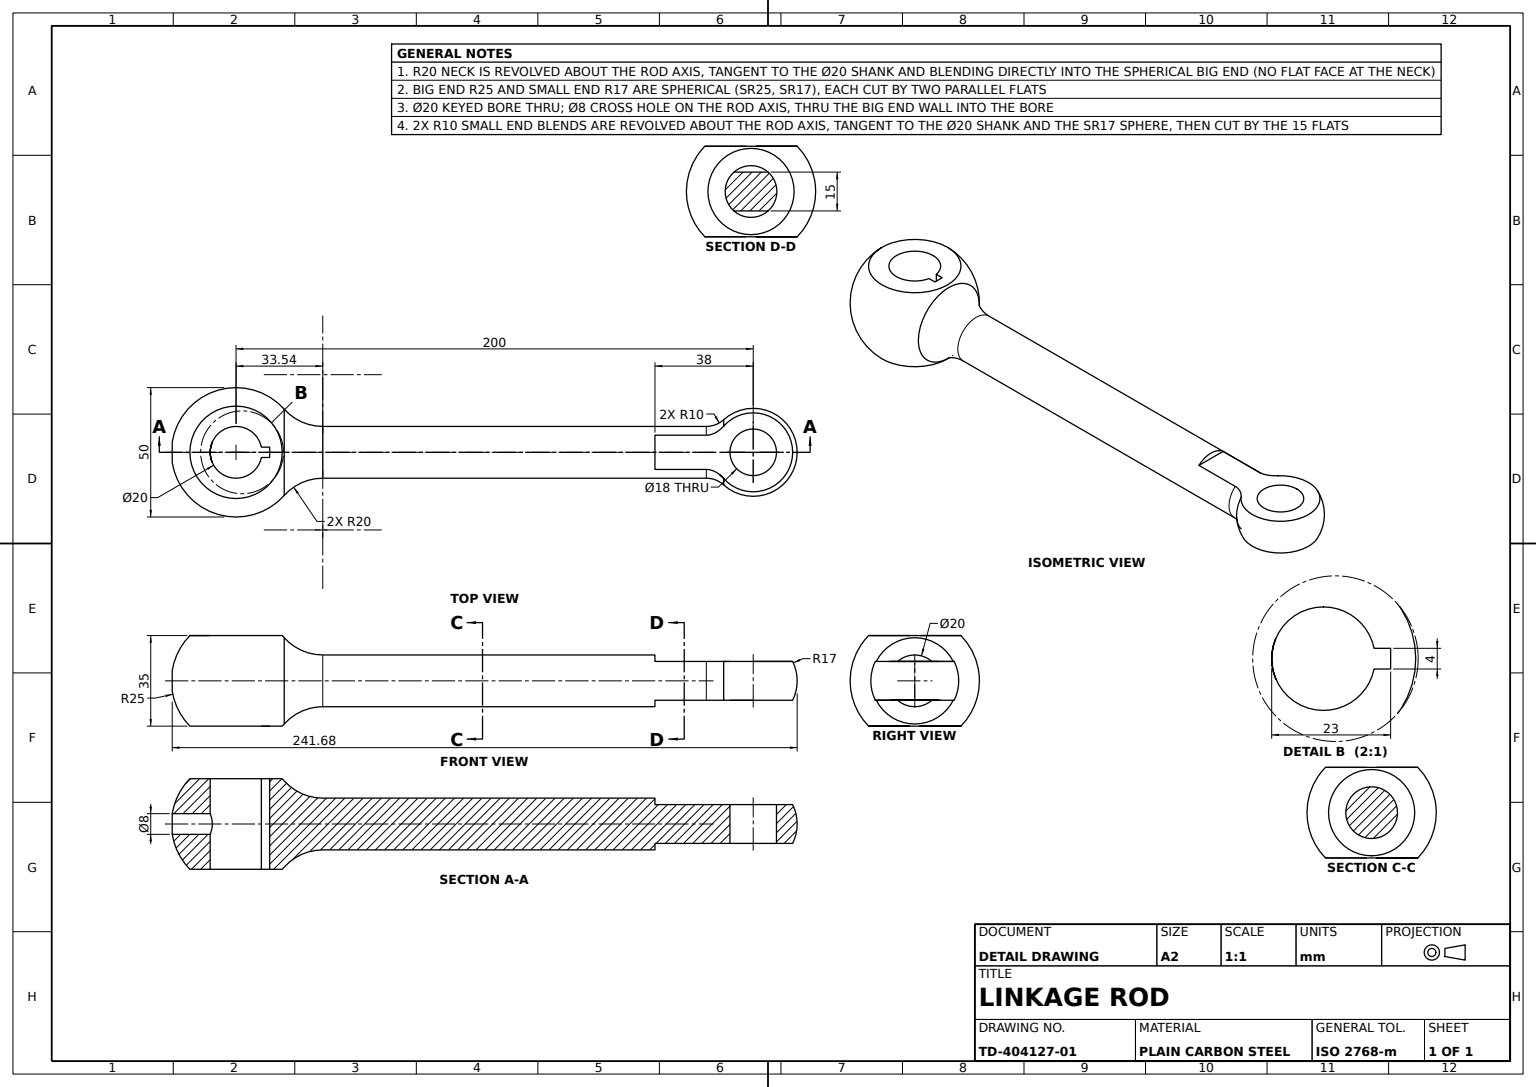
from build123d import *

# Parameters (mm, degrees)
SMALL_END_FLAT_DEPTH    = 10
BIG_END_FLAT_SKETCH_W   = 86.980428418
BIG_END_FLAT_SKETCH_H   = 55.493296348
BIG_END_FLAT_DEPTH      = 10
KEYED_BORE_20_DEPTH     = 40
SMALL_END_HOLE_SKETCH_R = 9
SMALL_END_HOLE_DEPTH    = 40
FILLET_R20_R            = 20
FILLET_R10_R            = 10
CROSS_HOLE_SKETCH_R     = 4
CROSS_HOLE_8_DEPTH      = 20


with BuildPart() as part:
    # Rod Profile Sketch → Rod Body Revolve (revolve)
    with BuildSketch(Plane.XY):
        with BuildLine():
            Line((-2.087121525, 10), (161.252272915, 10))
            ThreePointArc((161.252272915, 10), (180.257786585, 16.1664987), (192, 0))
            Line((192, 0), (-50, 0))
            ThreePointArc((-50, 0), (-30.107741092, 24.472657823), (-2.087121525, 10))
        make_face()
    revolve(axis=Axis((0, 0, 0), (1, 0, 0)))

    # Small End Flat Sketch → Small End Flat (cut)
    with BuildSketch(Plane(origin=(0, 7.5, 0), x_dir=(1, 0, 0), z_dir=(0, 1, 0))):
        Polygon((137.002179541, 20.26941877), (137.002179541, -16.521174788), (192.002179541, -16.521174788), (192.002179541, 18.008544306), align=None)
    small_end_flat = extrude(amount=SMALL_END_FLAT_DEPTH, mode=Mode.SUBTRACT)

    # Small End Flat Mirror: Small End Flat across plane
    add(small_end_flat.mirror(Plane.ZX), mode=Mode.SUBTRACT)

    # Big End Flat Sketch → Big End Flat (cut)
    with BuildSketch(Plane(origin=(0, 17.5, 0), x_dir=(1, 0, 0), z_dir=(0, 1, 0))):
        with Locations((-25, 0)):
            Rectangle(BIG_END_FLAT_SKETCH_W, BIG_END_FLAT_SKETCH_H)
    big_end_flat = extrude(amount=BIG_END_FLAT_DEPTH, mode=Mode.SUBTRACT)

    # Big End Flat Mirror: Big End Flat across plane
    add(big_end_flat.mirror(Plane.ZX), mode=Mode.SUBTRACT)

    # Keyed Bore Sketch → Keyed Bore Ø20 (cut)
    with BuildSketch(Plane(origin=(0, 17.5, 0), x_dir=(1, 0, 0), z_dir=(0, 1, 0))):
        with BuildLine():
            Line((-15.202041029, 2), (-12, 2))
            Line((-12, 2), (-12, -2))
            Line((-12, -2), (-15.202041029, -2))
            ThreePointArc((-15.202041029, -2), (-35, 0), (-15.202041029, 2))
        make_face()
    extrude(amount=-KEYED_BORE_20_DEPTH, mode=Mode.SUBTRACT)

    # Small End Hole Sketch → Small End Hole (cut)
    with BuildSketch(Plane(origin=(0, 7.5, 0), x_dir=(1, 0, 0), z_dir=(0, 1, 0))):
        with Locations(Location((175, 0, 0), (0, 0, 270))):
            Circle(SMALL_END_HOLE_SKETCH_R)
    extrude(amount=-SMALL_END_HOLE_DEPTH, mode=Mode.SUBTRACT)

    # Fillet R20
    fillet_r20_edges = [part.edges().sort_by_distance(p)[0] for p in [
        (-2.087121525, -10, 0),
    ]]
    fillet(fillet_r20_edges, radius=FILLET_R20_R)

    # Fillet R10
    fillet_r10_edges = [part.edges().sort_by_distance(p)[0] for p in [
        (161.252272915, 0, -10),
        (161.252272915, 0, 10),
    ]]
    fillet(fillet_r10_edges, radius=FILLET_R10_R)

    # Cross Hole Sketch → Cross Hole Ø8 (cut)
    with BuildSketch(Plane(origin=(-50, 0, 0), x_dir=(0, 0, -1), z_dir=(1, 0, 0))):
        with Locations(Location((0, 0, 0), (0, 0, 180))):
            Circle(CROSS_HOLE_SKETCH_R)
    extrude(amount=CROSS_HOLE_8_DEPTH, mode=Mode.SUBTRACT)


solid = part.part
